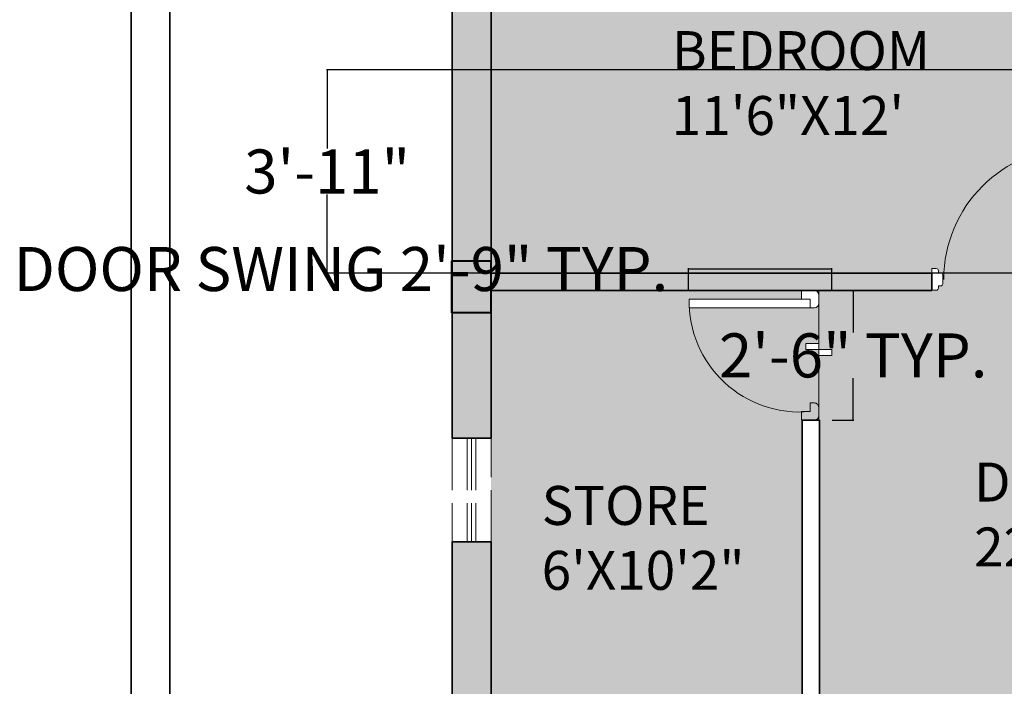
# Model space of a CAD drawing. Units: inches. Extents: x 1077 to 2505, y 1892 to 2728.
# Tile 11 of 26: x 1078 to 1306, y 2338 to 2492. Entities that reach past the tile are written whole.
import ezdxf

# ---------------------------------------------------------------- set-up
doc = ezdxf.new("R2010")
doc.units = ezdxf.units.IN
doc.linetypes.add('ACAD_ISO02W100', pattern=[15, 12, -3])
doc.layers.get('Defpoints').update_dxf_attribs({"color": 220, "linetype": 'ACAD_ISO02W100'})
for name, color, linetype, lineweight in [('00 FURNITURE', 15, 'Continuous', 15), ('A-ANNO-DIMS', 2, 'Continuous', 18), ('A-ANNO-TTLB', 7, 'Continuous', 35), ('A-AREA-IDEN', 7, 'Continuous', 18), ('A-COLS', 7, 'Continuous', 40), ('A-DOOR', 4, 'Continuous', 18), ('A-GLAZ-VENT', 6, 'ACAD_ISO02W100', 13), ('A-WALL-PATT', 7, 'Continuous', 9), ('A_FUR 1', 5, 'Continuous', 5), ('WALL', 7, 'Continuous', 35)]:
    doc.layers.add(name, color=color, linetype=linetype, lineweight=lineweight)
doc.layers.add('A-FLOR-PATT', color=254, linetype='Continuous', lineweight=9, true_color=0xd7ebd2)
doc.styles.get("Standard").update_dxf_attribs({"font": 'arial.ttf'})
doc.dimstyles.get("Standard").update_dxf_attribs({"dimtxt": 10.18, "dimasz": 0.18, "dimexe": 0.18, "dimexo": 0.0625, "dimgap": 0.09, "dimtad": 0, "dimtih": 1, "dimtoh": 1, "dimdec": 0, "dimzin": 0, "dimdsep": 46, "dimlunit": 3, "dimtxsty": 'Standard', "dimcen": 0.09, "dimadec": 0, "dimazin": 0, "dimtfac": 1, "dimtdec": 0, "dimtofl": 0, "dimtmove": 0, "dimatfit": 3, "dimfxl": 1, "dimtolj": 1, "dimtzin": 0, "dimarcsym": 0})

# ---------------------------------------------------------------- blocks, each defined once
blk = doc.blocks.new('DDD')
at = {"layer": '00 FURNITURE'}
for p, q in [((-12579.77, -15859.53), (-12579.77, -15829.05)), ((-12578.77, -15859.53), (-12578.77, -15829.03)), ((-12612.02, -15857.03), (-12612.02, -15862.03)), ((-12611.02, -15857.03), (-12612.02, -15857.03)), ((-12577.02, -15857.03), (-12576.02, -15857.03)), ((-12576.02, -15857.03), (-12576.02, -15862.03)), ((-12610.52, -15858.03), (-12610.52, -15857.53)), ((-12578.77, -15859.53), (-12579.77, -15859.53)), ((-12577.52, -15858.03), (-12577.52, -15857.53)), ((-12610.52, -15861.53), (-12610.52, -15861.03)), ((-12577.52, -15861.53), (-12577.52, -15861.03)), ((-12612.02, -15862.03), (-12611.02, -15862.03)), ((-12576.02, -15862.03), (-12577.02, -15862.03))]:
    blk.add_line(p, q, dxfattribs=at)
for points in [[(-12610.52, -15861.03), (-12610.02, -15861.03, 0.414214), (-12609.52, -15860.53), (-12609.52, -15858.53, 0.414214), (-12610.02, -15858.03), (-12610.52, -15858.03)], [(-12577.52, -15861.03), (-12578.02, -15861.03, -0.414214), (-12578.52, -15860.53), (-12578.52, -15858.53, -0.414214), (-12578.02, -15858.03), (-12577.52, -15858.03)]]:
    blk.add_lwpolyline(points, format="xyb", dxfattribs=at)
for centre, radius, start, end in [((-12578.77, -15859.53), 30.5, 90, 180), ((-12611.02, -15857.53), 0.5, 0, 90), ((-12577.02, -15857.53), 0.5, 90, 180), ((-12611.02, -15861.53), 0.5, 270, 0), ((-12577.02, -15861.53), 0.5, 180, 270)]:
    blk.add_arc(centre, radius, start, end, dxfattribs=at)
blk = doc.blocks.new('ESTSET')
at = {"layer": 'A_FUR 1'}
for p, q in [((-10.44, 4.1), (-10.44, 32.1)), ((-8.44, 4.1), (-8.44, 32.1)), ((-36.44, 6.1), (-36.44, 3.1)), ((-34.44, 6.1), (-36.44, 6.1)), ((-34.44, 4.1), (-34.44, 6.1)), ((-34.44, 4.1), (-34.44, 6.1)), ((-8.44, 4.1), (-8.44, 6.1)), ((-8.44, 6.1), (-6.44, 6.1)), ((-8.44, 4.1), (-8.44, 6.1)), ((-6.44, 6.1), (-6.44, 3.1)), ((-32.44, 4.1), (-34.44, 4.1)), ((-32.44, 4.1), (-34.44, 4.1)), ((-32.44, 3.1), (-32.44, 4.1)), ((-10.44, 3.1), (-10.44, 4.1)), ((-10.44, 4.1), (-8.44, 4.1)), ((-10.44, 4.1), (-8.44, 4.1)), ((-6.44, 2.1), (-36.44, 2.1)), ((-35.44, 2.1), (-33.44, 2.1)), ((-7.44, 2.1), (-9.44, 2.1))]:
    blk.add_line(p, q, dxfattribs=at)
for points in [[(-21.44, 2.1), (-18.67, 2.1), (-18.67, 5.1), (-20.06, 5.1)], [(-20.06, 5.1), (-20.06, -0.91)], [(-21.44, 2.1), (-21.44, -0.91), (-20.06, -0.91)]]:
    blk.add_lwpolyline(points, dxfattribs=at)
for centre, radius, start, end in [((-8.91, 6.46), 25.64, 88.9606, 185.2816), ((-35.44, 3.1), 1, 180, 270), ((-33.44, 3.1), 1, 270, 0), ((-9.44, 3.1), 1, 180, 270), ((-7.44, 3.1), 1, 270, 0)]:
    blk.add_arc(centre, radius, start, end, dxfattribs=at)
blk = doc.blocks.new('C1')
h = blk.add_hatch(color=256)
h.dxf.hatch_style = 1
h.paths.add_polyline_path([(1668.56, 2445.41), (1677.56, 2445.41), (1677.56, 2457.41), (1668.56, 2457.41)])
for p, q in [((1668.56, 2457.41), (1677.56, 2457.41)), ((1668.56, 2445.41), (1668.56, 2457.41)), ((1677.56, 2457.41), (1677.56, 2445.41)), ((1677.56, 2445.41), (1668.56, 2445.41))]:
    blk.add_line(p, q)
blk = doc.blocks.new('VENT-24')
for p, q in [((3.5, 24), (3.5, 0)), ((4.5, 24), (4.5, 0)), ((5.5, 24), (5.5, 0))]:
    blk.add_line(p, q)
blk.add_lwpolyline([(0, 0), (9, 0), (9, 24), (0, 24)], close=True)
blk = doc.blocks.new('SHEET-FRAME-RESIDENTIAL')
for points in [[(0, 830.04), (543.52, 830.04), (543.52, 0), (0, 0)], [(9, 821.04), (534.52, 821.04), (534.52, 9), (9, 9)]]:
    blk.add_lwpolyline(points, close=True)
blk = doc.blocks.new('*D34')
at = {"layer": 'A-ANNO-DIMS', "color": 0, "lineweight": -2, "transparency": 16777216}
for p, q in [((1233.24, 2434.11), (1233.06, 2434.11)), ((1233.24, 2429.21), (1233.24, 2434.29)), ((1266.19, 2434.11), (1233.42, 2434.11)), ((1266.37, 2429.21), (1266.37, 2434.29))]:
    blk.add_line(p, q, dxfattribs=at)
at = {"layer": 'A-ANNO-DIMS', "color": 0, "transparency": 16777216}
for points in [[(1233.42, 2434.14), (1233.42, 2434.08), (1233.24, 2434.11)], [(1266.19, 2434.14), (1266.19, 2434.08), (1266.37, 2434.11)]]:
    blk.add_solid(points, dxfattribs=at)
at = {"layer": 'Defpoints', "color": 0, "transparency": 16777216}
for p in [(1233.24, 2434.11), (1233.24, 2429.14), (1266.37, 2429.14)]:
    blk.add_point(p, dxfattribs=at)
at = {"layer": 'A-ANNO-DIMS', "color": 0, "transparency": 16777216, "insert": (1152.81, 2434.11), "char_height": 10.18, "attachment_point": 5}
blk.add_mtext('\\A1;DOOR SWING 2\'-9" TYP.', dxfattribs=at)
blk = doc.blocks.new('*D35')
at = {"layer": 'A-ANNO-DIMS', "color": 0, "lineweight": -2, "transparency": 16777216}
for p, q in [((1266.44, 2429.14), (1271.52, 2429.14)), ((1271.34, 2428.96), (1271.34, 2419.43)), ((1271.34, 2399.32), (1271.34, 2408.86)), ((1266.44, 2399.14), (1271.52, 2399.14))]:
    blk.add_line(p, q, dxfattribs=at)
at = {"layer": 'A-ANNO-DIMS', "color": 0, "transparency": 16777216}
for points in [[(1271.31, 2428.96), (1271.37, 2428.96), (1271.34, 2429.14)], [(1271.31, 2399.32), (1271.37, 2399.32), (1271.34, 2399.14)]]:
    blk.add_solid(points, dxfattribs=at)
at = {"layer": 'Defpoints', "color": 0, "transparency": 16777216}
for p in [(1266.37, 2429.14), (1271.34, 2429.14), (1266.37, 2399.14)]:
    blk.add_point(p, dxfattribs=at)
at = {"layer": 'A-ANNO-DIMS', "color": 0, "transparency": 16777216, "insert": (1271.34, 2414.14), "char_height": 10.18, "attachment_point": 5}
blk.add_mtext('\\A1;2\'-6" TYP.', dxfattribs=at)
blk = doc.blocks.new('*D64')
at = {"layer": 'A-ANNO-DIMS', "color": 0, "lineweight": -2, "transparency": 16777216}
for p, q in [((1395.47, 2480.16), (1149.43, 2480.16)), ((1149.61, 2479.98), (1149.61, 2461.95)), ((1149.61, 2433.34), (1149.61, 2451.37)), ((1395.47, 2433.16), (1149.43, 2433.16))]:
    blk.add_line(p, q, dxfattribs=at)
at = {"layer": 'A-ANNO-DIMS', "color": 0, "transparency": 16777216}
for points in [[(1149.58, 2479.98), (1149.64, 2479.98), (1149.61, 2480.16)], [(1149.58, 2433.34), (1149.64, 2433.34), (1149.61, 2433.16)]]:
    blk.add_solid(points, dxfattribs=at)
at = {"layer": 'Defpoints', "color": 0, "transparency": 16777216}
for p in [(1149.61, 2480.16), (1395.53, 2480.16), (1395.53, 2433.16)]:
    blk.add_point(p, dxfattribs=at)
at = {"layer": 'A-ANNO-DIMS', "color": 0, "transparency": 16777216, "insert": (1149.61, 2456.66), "char_height": 10.18, "attachment_point": 5}
blk.add_mtext('\\A1;3\'-11"', dxfattribs=at)

msp = doc.modelspace()

# ---------------------------------------------------------------- hatches: boundary and pattern name
at = {"layer": 'A-FLOR-PATT', "transparency": 33554559}
h = msp.add_hatch(color=256, dxfattribs=at)
h.dxf.hatch_style = 1
h.paths.add_polyline_path([(1395.53, 2577.16), (1374.83, 2577.16), (1350.83, 2577.19), (1350.83, 2577.16), (1329.53, 2577.16), (1329.53, 2480.16), (1329.53, 2469.16), (1325.53, 2469.16), (1325.53, 2515.13), (1307.53, 2515.13), (1307.53, 2577.16), (1269.31, 2577.16), (1221.31, 2577.15), (1221.31, 2577.16), (1187.53, 2577.16), (1187.53, 2433.16), (1289.53, 2433.16), (1289.53, 2429.16), (1263.53, 2429.16), (1187.53, 2429.16), (1187.53, 2395.02), (1187.53, 2395.02), (1187.53, 2371.02), (1187.53, 2371.02), (1187.53, 2307.16), (1259.53, 2307.16), (1259.53, 2399.16), (1263.53, 2399.16), (1263.53, 2307.16), (1289.53, 2307.16), (1289.53, 2306.23), (1325.53, 2306.23), (1325.53, 2307.16), (1329.53, 2307.16), (1329.53, 2306.23), (1365.53, 2306.23), (1365.53, 2307.16), (1432.53, 2307.16), (1432.53, 2088.16), (1547.53, 2088.16), (1547.53, 2140.08), (1511.53, 2140.08), (1511.53, 2267.16), (1475.53, 2267.16), (1475.53, 2303.16), (1468.53, 2303.16), (1468.53, 2307.16), (1547.53, 2307.16), (1547.53, 2348.22), (1547.53, 2396.22), (1547.53, 2429.16), (1435.53, 2429.16), (1435.53, 2433.16), (1476.35, 2433.16), (1476.35, 2451.18), (1547.53, 2451.18), (1547.53, 2577.16), (1499.53, 2577.16), (1499.53, 2586.16), (1547.53, 2586.16), (1547.53, 2642.16), (1518.18, 2642.16), (1518.18, 2642.05), (1494.15, 2642.05), (1494.15, 2642.16), (1469.53, 2642.16), (1469.53, 2577.16), (1399.53, 2577.16), (1399.53, 2429.16), (1325.53, 2429.16), (1325.53, 2433.16), (1329.53, 2433.16), (1395.53, 2433.16), (1395.53, 2480.16), (1359.53, 2480.16), (1359.53, 2484.16), (1395.53, 2484.16)])
h.paths.add_polyline_path([(1357.65, 2482.07), (1355.65, 2482.07), (1355.65, 2481.07, 0.414214), (1356.65, 2480.07), (1344.65, 2480.07), (1344.65, 2477.06), (1343.27, 2477.06), (1343.27, 2480.07), (1330.65, 2480.07, -0.414214), (1329.65, 2481.07), (1329.65, 2484.07), (1331.65, 2484.07), (1331.65, 2510.07, -0.446908)], flags=16)
h.paths.add_polyline_path([(1305.09, 2559.18), (1288.89, 2559.18), (1288.89, 2575.38), (1305.09, 2575.38)], flags=16)
h.paths.add_polyline_path([(1304.19, 2560.08), (1289.79, 2560.08), (1289.79, 2574.48), (1304.19, 2574.48)], flags=0)
h.paths.add_polyline_path([(1287.99, 2500.68, -0.414214), (1287.09, 2499.78), (1265.14, 2499.78), (1224.09, 2499.78, -0.414214), (1223.19, 2500.68), (1223.19, 2557.16), (1223.19, 2571.74), (1223.19, 2575.38), (1287.99, 2575.38), (1287.99, 2571.74), (1287.09, 2571.74, -0.414214), (1287.99, 2570.84)], flags=16)
h.paths.add_polyline_path([(1292.98, 2569.05, -1), (1300.92, 2569.05, -1)], flags=0)
h.paths.add_polyline_path([(1293.32, 2569.05, -1), (1300.58, 2569.05, -1)], flags=0)
h.paths.add_polyline_path([(1322.8, 2462.21), (1322.8, 2431.71), (1323.05, 2430.71), (1323.05, 2431.71), (1321.8, 2431.71), (1321.8, 2462.19, 0.404641), (1292.3, 2431.71), (1292.05, 2430.71, -0.414214), (1291.55, 2430.21), (1291.05, 2430.21), (1291.05, 2429.71, -0.414214), (1290.55, 2429.21), (1289.55, 2429.21), (1289.55, 2434.21), (1290.55, 2434.21, -0.414214), (1291.05, 2433.71), (1291.05, 2433.21), (1291.55, 2433.21, -0.414214), (1292.05, 2432.71), (1292.3, 2431.71, -0.414214)], flags=16)
h.paths.add_polyline_path([(1287.82, 2548.28, 0.292232), (1279.17, 2536.8, 0.052719), (1223.93, 2548.28), (1223.28, 2548.28), (1223.28, 2557.16), (1223.93, 2557.16), (1245.42, 2557.16, -0.117785), (1245.77, 2557.93, -0.059418), (1254.87, 2567.02, -0.379859), (1257.28, 2566.88, -0.02509), (1261.41, 2563.32, -0.025935), (1265.65, 2567.02, -0.379859), (1268.06, 2566.88, -0.061767), (1277.52, 2557.43, -0.069393), (1277.82, 2557.16), (1287.82, 2557.16)], flags=0)
h.paths.add_polyline_path([(1263.47, 2548.28), (1260.56, 2548.28, -0.015371), (1258.01, 2546.13, -0.429576), (1255.37, 2546.06, -0.016036), (1252.69, 2548.28), (1223.28, 2548.28), (1223.28, 2554.42), (1246.78, 2554.42, 0.055344), (1255.37, 2546.06, 0.331768), (1257.52, 2545.74, 0.027343), (1262, 2549.64, 0.00919)], flags=0)
h.paths.add_polyline_path([(1295.56, 2568.34), (1296.87, 2569.09), (1296.87, 2570.6, 0.399698), (1295.39, 2569.05, 0.119004)], flags=0)
h.paths.add_polyline_path([(1295.21, 2569.05, -1), (1298.68, 2569.05, -1)], flags=0)
h.paths.add_polyline_path([(1296.95, 2568.96), (1297.03, 2569), (1297.03, 2569.09), (1296.99, 2569.11), (1296.91, 2568.98)], flags=0)
h.paths.add_polyline_path([(1402.28, 2462.19, -0.414214), (1432.78, 2431.69), (1433.03, 2432.69), (1432.78, 2431.69, 0.404641), (1403.28, 2462.17), (1403.28, 2431.69), (1402.03, 2431.69), (1402.03, 2430.69, -0.414214), (1401.53, 2430.19), (1401.03, 2430.19), (1401.03, 2429.69, -0.414214), (1400.53, 2429.19), (1399.53, 2429.19), (1399.53, 2434.19), (1400.53, 2434.19, -0.414214), (1401.03, 2433.69), (1401.03, 2433.19), (1401.53, 2433.19, -0.414214), (1402.03, 2432.69)], flags=16)
h.paths.add_polyline_path([(1470.16, 2535.21, -0.414214), (1471.06, 2536.11), (1527.54, 2536.11), (1542.12, 2536.11), (1545.76, 2536.11), (1545.76, 2471.31), (1542.12, 2471.31), (1542.12, 2472.21, -0.414214), (1541.22, 2471.31), (1471.06, 2471.31, -0.414214), (1470.16, 2472.21), (1470.16, 2494.16)], flags=16)
h.paths.add_polyline_path([(1483.07, 2536.11, 0.253465), (1480.11, 2526.15, 0.2538), (1470.15, 2523.19)], flags=16)
h.paths.add_polyline_path([(1223.19, 2512.69, 0.253465), (1233.14, 2509.74, 0.2538), (1236.1, 2499.77)], flags=16)
h.paths.add_polyline_path([(1469.77, 2578.72), (1469.77, 2581.72), (1471.77, 2581.72), (1471.77, 2607.72, -0.01951), (1473.77, 2607.68), (1473.77, 2579.72), (1473.77, 2578.72, -0.414214), (1472.77, 2577.72), (1470.77, 2577.72, -0.414214)], flags=16)
h.paths.add_polyline_path([(1382.46, 2398.13), (1395.04, 2398.13), (1395.04, 2399.74), (1382.46, 2399.74)], flags=16)
h.paths.add_polyline_path([(1379.94, 2397.18), (1379.94, 2389.82), (1380.5, 2389.82), (1380.5, 2396.05, -0.41429), (1381.06, 2396.61), (1396.47, 2396.61, -0.414213), (1397.03, 2396.05), (1397.03, 2389.82), (1397.59, 2389.82), (1397.59, 2397.18)], flags=16)
h.paths.add_polyline_path([(1263.37, 2428.14), (1263.37, 2426.14, -0.414214), (1262.37, 2425.14), (1261.37, 2425.14), (1233.41, 2425.14, 0.400854), (1259.37, 2401.04), (1259.37, 2401.14), (1261.37, 2401.14, -0.446908), (1233.37, 2427.14), (1259.37, 2427.14), (1259.37, 2429.14), (1262.37, 2429.14, -0.414214)], flags=16)
h.paths.add_polyline_path([(1404.79, 2398.13), (1417.37, 2398.13), (1417.37, 2399.74), (1404.79, 2399.74)], flags=16)
h.paths.add_polyline_path([(1402.27, 2397.18), (1404.79, 2398.13), (1417.37, 2398.13), (1419.92, 2397.18)], flags=16)
h.paths.add_polyline_path([(1432.26, 2383.16), (1432.26, 2370.59), (1433.87, 2370.59), (1433.87, 2383.16)], flags=16)
h.paths.add_polyline_path([(1431.3, 2385.69), (1423.84, 2385.69), (1423.84, 2385.13), (1430.18, 2385.13, -0.41429), (1430.74, 2384.57), (1430.74, 2369.16, -0.414237), (1430.18, 2368.6), (1423.84, 2368.6), (1423.84, 2368.03), (1431.3, 2368.03)], flags=16)
h.paths.add_polyline_path([(1417.37, 2351.16), (1417.37, 2349.54), (1418.9, 2349.54, 0.414236), (1419.92, 2350.56), (1419.92, 2352.11)], flags=16)
h.paths.add_polyline_path([(1395.04, 2351.16), (1395.04, 2349.54), (1396.58, 2349.54, 0.414235), (1397.59, 2350.56), (1397.59, 2352.11)], flags=16)
h.paths.add_polyline_path([(1366.7, 2370.05), (1365.09, 2370.05), (1365.09, 2368.52, 0.414235), (1366.11, 2367.5), (1367.66, 2367.5)], flags=16)
h.paths.add_polyline_path([(1419.36, 2359.47), (1419.36, 2353.24, -0.41419), (1418.8, 2352.68), (1403.39, 2352.68, -0.414137), (1402.83, 2353.24), (1402.83, 2359.47), (1397.03, 2359.47), (1397.03, 2353.24, -0.414189), (1396.47, 2352.68), (1381.06, 2352.68, -0.414137), (1380.5, 2353.24), (1380.5, 2359.47)], flags=16)
h.paths.add_polyline_path([(1222.29, 2559.18), (1206.09, 2559.18), (1206.09, 2575.38), (1222.29, 2575.38)], flags=16)
h.paths.add_polyline_path([(1221.39, 2560.08), (1206.99, 2560.08), (1206.99, 2574.48), (1221.39, 2574.48)], flags=0)
h.paths.add_polyline_path([(1482, 2577.72), (1482, 2580.73), (1483.38, 2580.73), (1483.38, 2577.72), (1484.77, 2577.72), (1484.77, 2574.72), (1483.38, 2574.72), (1483.38, 2577.72)], flags=16)
h.paths.add_polyline_path([(1266.37, 2415.53), (1266.37, 2414.14), (1263.37, 2414.14), (1263.37, 2415.53), (1260.36, 2415.53), (1260.36, 2416.91), (1263.37, 2416.91), (1263.37, 2415.53)], flags=16)
h.paths.add_polyline_path([(1210.26, 2569.05, -1), (1218.19, 2569.05, -1)], flags=0)
h.paths.add_polyline_path([(1210.6, 2569.05, -1), (1217.85, 2569.05, -1)], flags=0)
h.paths.add_polyline_path([(1212.84, 2568.34), (1214.15, 2569.09), (1214.15, 2570.6, 0.399698), (1212.67, 2569.05, 0.119004)], flags=0)
h.paths.add_polyline_path([(1212.49, 2569.05, -1), (1215.96, 2569.05, -1)], flags=0)
h.paths.add_polyline_path([(1214.23, 2568.96), (1214.3, 2568.91), (1214.3, 2569)], flags=0)
h.paths.add_polyline_path([(1507.18, 2480.12, 0.052719), (1518.66, 2535.36), (1518.66, 2536.01), (1527.54, 2536.01), (1527.54, 2535.36), (1527.54, 2513.88, -0.117785), (1528.31, 2513.53, -0.059418), (1537.4, 2504.43, -0.379859), (1537.26, 2502.01, -0.02509), (1533.7, 2497.89, -0.025935), (1537.4, 2493.64, -0.379859), (1537.26, 2491.23, -0.061767), (1527.8, 2481.77, -0.069393), (1527.54, 2481.47), (1527.54, 2471.47), (1518.66, 2471.47, 0.292232)], flags=0)
h.paths.add_polyline_path([(1516.43, 2503.92, -0.016036), (1518.66, 2506.6), (1518.66, 2536.01), (1524.8, 2536.01), (1524.8, 2512.51, 0.055344), (1516.43, 2503.92, 0.331768), (1516.12, 2501.77, 0.027343), (1520.01, 2497.29, 0.00919), (1518.66, 2495.82), (1518.66, 2498.73, -0.015371), (1516.5, 2501.28, -0.429576)], flags=0)
h.paths.add_polyline_path([(1499.63, 2625.5, -0.171636), (1502.82, 2631.01), (1502.82, 2633.37), (1498.68, 2633.37, -0.414214), (1497.7, 2634.36), (1497.7, 2640.66, -0.414214), (1498.68, 2641.64), (1514.82, 2641.64, -0.414214), (1515.81, 2640.66), (1515.81, 2634.36, -0.414214), (1514.82, 2633.37), (1510.69, 2633.37), (1510.69, 2631.01, -0.171636), (1513.88, 2625.5, -0.258205), (1509.31, 2614.47), (1504.19, 2614.47, -0.258205)], flags=16)
h.paths.add_polyline_path([(1501.2, 2625.5, -0.171636), (1504.39, 2631.01), (1509.12, 2631.01, -0.171636), (1512.3, 2625.5, -0.210384), (1509.35, 2616.02), (1504.16, 2616.02, -0.210384)], flags=0)
h.paths.add_polyline_path([(1529.56, 2537.01), (1529.56, 2553.21), (1545.76, 2553.21), (1545.76, 2537.01)], flags=16)
h.paths.add_polyline_path([(1530.46, 2537.91), (1530.46, 2552.31), (1544.86, 2552.31), (1544.86, 2537.91)], flags=0)
h.paths.add_polyline_path([(1535.45, 2545.07, -1), (1543.39, 2545.07, -1)], flags=0)
h.paths.add_polyline_path([(1535.8, 2545.07, -1), (1543.05, 2545.07, -1)], flags=0)
h.paths.add_polyline_path([(1529.56, 2470.41), (1545.76, 2470.41), (1545.76, 2454.21), (1529.56, 2454.21)], flags=16)
h.paths.add_polyline_path([(1541.16, 2544.99), (1540.98, 2544.99, -0.544606), (1538.71, 2543.68), (1538.62, 2543.53, 0.547962)], flags=0)
h.paths.add_polyline_path([(1530.46, 2469.51), (1544.86, 2469.51), (1544.86, 2455.11), (1530.46, 2455.11)], flags=0)
h.paths.add_polyline_path([(1539.47, 2545.14), (1539.42, 2545.22), (1539.38, 2545.14)], flags=0)
h.paths.add_polyline_path([(1543.39, 2462.34, -1), (1535.45, 2462.34, -1)], flags=0)
h.paths.add_polyline_path([(1543.05, 2462.34, -1), (1535.8, 2462.34, -1)], flags=0)
h.paths.add_polyline_path([(1541.16, 2462.27), (1540.98, 2462.27, -0.544606), (1538.71, 2460.96), (1538.62, 2460.8, 0.547962)], flags=0)
h.paths.add_polyline_path([(1539.47, 2462.42), (1539.42, 2462.5), (1539.38, 2462.42)], flags=0)
h.paths.add_polyline_path([(1435.32, 2335.25, -0.414214), (1465.82, 2304.75), (1466.07, 2305.75), (1465.82, 2304.75, 0.404641), (1436.32, 2335.23), (1436.32, 2304.75), (1435.07, 2304.75), (1435.07, 2303.75, -0.414214), (1434.57, 2303.25), (1434.07, 2303.25), (1434.07, 2302.75, -0.414214), (1433.57, 2302.25), (1432.57, 2302.25), (1432.57, 2307.25), (1433.57, 2307.25, -0.414214), (1434.07, 2306.75), (1434.07, 2306.25), (1434.57, 2306.25, -0.414214), (1435.07, 2305.75)], flags=16)
h.paths.add_polyline_path([(1532.13, 2635.71), (1535.43, 2635.71), (1535.43, 2635.89), (1532.13, 2635.89)], flags=16)
edge = h.paths.add_edge_path(flags=16)
edge.add_arc((1535.98, 2632.67), 0.183, 270, 360)
edge.add_line((1536.17, 2632.67), (1536.17, 2639.82))
edge.add_line((1536.17, 2639.82), (1538.29, 2639.82))
edge.add_line((1538.29, 2639.82), (1538.29, 2641.82))
edge.add_line((1538.29, 2641.82), (1533.25, 2641.82))
edge.add_line((1533.25, 2641.82), (1533.25, 2639.82))
edge.add_line((1533.25, 2639.82), (1534.87, 2639.82))
edge.add_line((1534.87, 2639.82), (1534.87, 2639))
edge.add_line((1534.87, 2639), (1533.7, 2639))
edge.add_line((1533.7, 2639), (1533.7, 2639.82))
edge.add_line((1533.7, 2639.82), (1533.25, 2639.82))
edge.add_line((1533.25, 2639.82), (1533.25, 2641.82))
edge.add_line((1533.25, 2641.82), (1538.29, 2641.82))
edge.add_line((1538.29, 2641.82), (1538.29, 2641.34))
edge.add_line((1538.29, 2641.34), (1540.64, 2641.58))
edge.add_line((1540.64, 2641.58), (1540.64, 2641.82))
edge.add_line((1540.64, 2641.82), (1541.5, 2641.82))
edge.add_line((1541.5, 2641.82), (1541.5, 2641.25))
edge.add_line((1541.5, 2641.25), (1541.31, 2639.79))
edge.add_ellipse((1541.09, 2638.95), major_axis=(-1.08, 0), ratio=0.790849, start_angle=180, end_angle=255.2976, ccw=False)
edge.add_line((1542.17, 2638.95), (1542.17, 2638.38))
edge.add_ellipse((1541.09, 2638.38), major_axis=(-1.08, 0), ratio=0.790849, start_angle=0, end_angle=180, ccw=False)
edge.add_line((1540, 2638.38), (1540.01, 2638.87))
edge.add_ellipse((1541.09, 2638.95), major_axis=(-1.08, 0), ratio=0.790849, start_angle=284.7024, end_angle=364.0401, ccw=False)
edge.add_line((1540.78, 2639.75), (1540.78, 2641.25))
edge.add_line((1540.78, 2641.25), (1540.64, 2641.25))
edge.add_line((1540.64, 2641.25), (1538.29, 2641.01))
edge.add_line((1538.29, 2641.01), (1538.29, 2639.82))
edge.add_line((1538.29, 2639.82), (1536.17, 2639.82))
edge.add_line((1536.17, 2639.82), (1536.17, 2632.48))
edge.add_line((1536.17, 2632.48), (1535.98, 2632.48))
h.paths.add_polyline_path([(1496.32, 2250.34, -0.292371), (1498.9, 2247.83, -0.085148), (1501.21, 2208.85, -0.01331), (1500.27, 2098.5, -0.379287), (1497.22, 2095.28, -0.0502), (1441.54, 2095.28, -0.379287), (1438.5, 2098.5, -0.01331), (1437.56, 2208.85, -0.086132), (1439.96, 2248.26, -0.295116), (1442.59, 2250.78, -0.114238)], flags=16)
h.paths.add_polyline_path([(1495.16, 2205.84, -0.355389), (1496.7, 2202.1), (1492.94, 2189.65, -0.398275), (1489.12, 2187.47, 0.113332), (1449.64, 2187.47, -0.398275), (1445.82, 2189.65), (1442.06, 2202.1, -0.355394), (1443.6, 2205.84, -0.265725)], flags=0)
h.paths.add_polyline_path([(1440.37, 2195.72), (1445.94, 2181.67), (1445.94, 2160.63), (1440.84, 2157.26)], flags=0)
h.paths.add_polyline_path([(1498.46, 2195.72), (1497.99, 2157.26), (1492.88, 2160.63), (1492.88, 2181.67)], flags=0)
h.paths.add_polyline_path([(1445.94, 2158.37), (1445.94, 2137.12), (1441.12, 2122.56), (1440.87, 2155.03)], flags=0)
h.paths.add_polyline_path([(1492.88, 2158.37), (1497.96, 2155.03), (1497.71, 2122.56), (1492.88, 2137.12)], flags=0)
h.paths.add_polyline_path([(1489.88, 2130.4), (1494.39, 2107.67, -0.090102), (1444.44, 2107.65), (1448.95, 2130.39, 0.036636)], flags=0)
h.paths.add_polyline_path([(1447.54, 2159.34), (1497.44, 2159.34), (1497.44, 2177.89), (1447.54, 2177.89)], flags=8)
h.paths.add_polyline_path([(1196.44, 2354.84), (1246.65, 2354.84), (1246.65, 2388.43), (1196.44, 2388.43)], flags=24)
h.paths.add_polyline_path([(1296.09, 2360.25), (1353.81, 2360.25), (1353.81, 2393.84), (1296.09, 2393.84)], flags=24)
h.paths.add_polyline_path([(1400.72, 2471.85), (1470.63, 2471.85), (1470.63, 2505.44), (1400.72, 2505.44)], flags=24)
h.paths.add_polyline_path([(1324.78, 2448.48), (1394.95, 2448.48), (1394.95, 2467.02), (1324.78, 2467.02)], flags=24)
h.paths.add_polyline_path([(1335.08, 2531.43), (1389.67, 2531.43), (1389.67, 2565.02), (1335.08, 2565.02)], flags=24)
h.paths.add_polyline_path([(1225.76, 2460), (1295.67, 2460), (1295.67, 2493.58), (1225.76, 2493.58)], flags=24)
h = msp.add_hatch(color=256, dxfattribs=at)
h.dxf.hatch_style = 1
h.paths.add_polyline_path([(1547.53, 2348.22), (1547.53, 2396.22), (1547.53, 2425.11), (1547.53, 2425.11), (1547.53, 2429.16), (1435.53, 2429.16), (1434.03, 2429.21), (1434.03, 2430.19), (1433.03, 2430.19), (1432.78, 2431.69, 0.404641), (1403.28, 2462.17), (1403.28, 2431.69), (1402.03, 2431.69), (1402.03, 2430.19), (1401.03, 2430.19), (1401.03, 2429.19), (1399.53, 2429.19), (1399.53, 2429.19), (1399.53, 2429.16), (1334.67, 2429.16), (1334.67, 2423.95), (1325.67, 2423.95), (1325.67, 2429.16), (1325.53, 2429.16), (1324.05, 2429.24), (1324.05, 2430.21), (1323.05, 2430.21), (1323.05, 2431.71), (1321.8, 2431.71), (1321.8, 2462.19, 0.416544), (1292.05, 2430.73, -0.423614), (1291.55, 2430.21), (1291.05, 2430.21), (1291.05, 2429.21), (1289.55, 2429.21), (1289.53, 2429.21), (1289.53, 2429.16), (1263.37, 2429.16), (1263.37, 2415.53), (1266.37, 2415.53), (1266.37, 2414.14), (1263.37, 2414.14), (1263.37, 2399.16), (1263.53, 2399.16), (1263.53, 2307.16), (1289.53, 2307.16), (1289.53, 2306.23), (1323.26, 2306.23), (1323.26, 2307.21), (1332.26, 2307.21), (1365.53, 2306.23), (1365.53, 2307.16), (1432.53, 2307.16), (1432.57, 2307.16), (1432.57, 2307.25), (1434.07, 2307.25), (1434.07, 2306.25), (1435.32, 2306.25), (1435.32, 2335.25, -0.407346), (1466.07, 2305.73, -0.423614), (1466.57, 2306.25), (1467.07, 2306.25), (1467.07, 2307.25), (1468.57, 2307.25), (1547.53, 2307.16), (1547.53, 2307.2)])
h.paths.add_polyline_path([(1430.74, 2369.16), (1430.74, 2384.57, 0.41429), (1430.18, 2385.13), (1423.84, 2385.13), (1423.84, 2368.6), (1430.18, 2368.6, 0.414237)], flags=16)
h.paths.add_polyline_path([(1432.26, 2383.16), (1432.26, 2370.59), (1433.87, 2370.59), (1433.87, 2383.16)], flags=16)
h.paths.add_polyline_path([(1431.3, 2368.03), (1431.3, 2385.69), (1432.26, 2383.16), (1432.26, 2370.59)], flags=16)
h.paths.add_polyline_path([(1417.37, 2351.16), (1417.37, 2349.54), (1418.9, 2349.54, 0.414236), (1419.92, 2350.56), (1419.92, 2352.11)], flags=16)
h.paths.add_polyline_path([(1403.39, 2352.68), (1418.78, 2352.68, 0.42427), (1419.36, 2353.24), (1419.36, 2359.47), (1402.83, 2359.47), (1402.83, 2353.24, 0.414137)], flags=16)
h.paths.add_polyline_path([(1366.7, 2370.05), (1365.09, 2370.05), (1365.09, 2368.52, 0.414235), (1366.11, 2367.5), (1367.66, 2367.5)], flags=16)
h.paths.add_polyline_path([(1382.46, 2398.13), (1395.04, 2398.13), (1395.04, 2399.74), (1382.46, 2399.74)], flags=16)
h.paths.add_polyline_path([(1396.47, 2396.61), (1381.06, 2396.61, 0.41429), (1380.5, 2396.05), (1380.5, 2389.82), (1397.03, 2389.82), (1397.03, 2396.05, 0.414213)], flags=16)
h.paths.add_polyline_path([(1402.27, 2397.18), (1402.83, 2396.05, -0.414213), (1403.39, 2396.61)], flags=16)
h.paths.add_polyline_path([(1418.8, 2396.61), (1419.36, 2396.61), (1419.36, 2396.05, 0.414237)], flags=16)
h.paths.add_polyline_path([(1404.79, 2398.13), (1417.37, 2398.13), (1417.37, 2399.74), (1404.79, 2399.74)], flags=16)
h.paths.add_polyline_path([(1381.06, 2352.68, -0.414213), (1380.5, 2353.24), (1380.27, 2352.11)], flags=16)
h.paths.add_polyline_path([(1396.58, 2349.54), (1396.58, 2349.54), (1395.04, 2349.54), (1395.04, 2349.54), (1382.46, 2349.54), (1382.46, 2351.16), (1395.04, 2351.16), (1397.59, 2352.11), (1397.59, 2350.56, -0.414235)], flags=16)
h.paths.add_polyline_path([(1379.94, 2397.18), (1382.46, 2398.13), (1395.04, 2398.13), (1397.59, 2397.18)], flags=16)
h.paths.add_polyline_path([(1368.78, 2384.59, 0.414213), (1368.22, 2384.03), (1367.66, 2367.5), (1367.66, 2385.15)], flags=16)
h.paths.add_polyline_path([(1547.53, 2574.38), (1547.51, 2574.38), (1547.51, 2577.16), (1499.53, 2577.16), (1484.77, 2577.44), (1484.77, 2574.72), (1483.38, 2574.72), (1483.38, 2577.72), (1482, 2577.72), (1469.53, 2577.72), (1469.53, 2577.16), (1401.95, 2577.16), (1401.95, 2574.12), (1399.53, 2574.12), (1399.53, 2434.19), (1401.03, 2434.19), (1401.03, 2433.19), (1402.28, 2433.19), (1402.28, 2462.19, -0.407346), (1433.03, 2432.67, -0.423614), (1433.53, 2433.19), (1434.03, 2433.19), (1434.03, 2434.19), (1435.53, 2434.19), (1476.35, 2433.81), (1476.35, 2451.18), (1547.53, 2451.18)])
h.paths.add_polyline_path([(1470.16, 2535.21, -0.414214), (1471.06, 2536.11), (1527.54, 2536.11), (1542.12, 2536.11), (1545.76, 2536.11), (1545.76, 2471.31), (1542.12, 2471.31), (1542.12, 2472.21, -0.414214), (1541.22, 2471.31), (1471.06, 2471.31, -0.414214), (1470.16, 2472.21), (1470.16, 2494.16)], flags=16)
h.paths.add_polyline_path([(1483.07, 2536.11, 0.253465), (1480.11, 2526.15, 0.2538), (1470.15, 2523.19)], flags=16)
h.paths.add_polyline_path([(1525.55, 2481.52, -0.000893), (1524.8, 2482.24), (1524.8, 2471.47), (1527.54, 2471.47), (1527.54, 2472.12), (1527.54, 2481.47, -0.388819)], flags=0)
h.paths.add_polyline_path([(1518.66, 2536.01), (1527.54, 2536.01), (1527.54, 2535.36), (1527.54, 2513.88, -0.117785), (1528.31, 2513.53, -0.059418), (1537.4, 2504.43, -0.379859), (1537.26, 2502.01, -0.02509), (1533.7, 2497.89, 0.033431), (1528.3, 2502.74, 0.308459), (1526.25, 2502.88, 0.047827), (1518.66, 2495.82), (1518.66, 2498.73, -0.015371), (1516.5, 2501.28, -0.429576), (1516.43, 2503.92, -0.016036), (1518.66, 2506.6)], flags=0)
h.paths.add_polyline_path([(1529.56, 2537.01), (1529.56, 2553.21), (1545.76, 2553.21), (1545.76, 2537.01)], flags=16)
h.paths.add_polyline_path([(1530.46, 2537.91), (1530.46, 2552.31), (1544.86, 2552.31), (1544.86, 2537.91)], flags=0)
h.paths.add_polyline_path([(1535.8, 2545.07, -1), (1543.05, 2545.07, -1)], flags=0)
h.paths.add_polyline_path([(1541.16, 2544.99), (1540.98, 2544.99, -0.544606), (1538.71, 2543.68), (1538.62, 2543.53, 0.547962)], flags=0)
h.paths.add_polyline_path([(1539.47, 2545.14), (1539.42, 2545.22), (1539.38, 2545.14)], flags=0)
h.paths.add_polyline_path([(1529.56, 2470.41), (1545.76, 2470.41), (1545.76, 2454.21), (1529.56, 2454.21)], flags=16)
h.paths.add_polyline_path([(1530.46, 2469.51), (1544.86, 2469.51), (1544.86, 2455.11), (1530.46, 2455.11)], flags=0)
h.paths.add_polyline_path([(1535.8, 2462.34, -1), (1543.05, 2462.34, -1)], flags=0)
h.paths.add_polyline_path([(1541.16, 2462.27), (1540.98, 2462.27, -0.544606), (1538.71, 2460.96), (1538.62, 2460.8, 0.547962)], flags=0)
h.paths.add_polyline_path([(1539.47, 2462.42), (1539.42, 2462.5), (1539.38, 2462.42)], flags=0)
h.paths.add_polyline_path([(1395.53, 2574.12), (1392.95, 2574.12), (1392.95, 2577.16), (1374.83, 2577.16), (1350.83, 2577.19), (1350.83, 2577.16), (1332.07, 2577.16), (1332.07, 2574), (1329.53, 2574), (1329.53, 2484.07), (1331.65, 2484.07), (1331.65, 2510.07, -0.423677), (1357.76, 2484.07), (1359.53, 2484.07), (1359.53, 2484.16), (1395.53, 2484.16)], flags=17)
h.paths.add_polyline_path([(1395.53, 2480.16), (1359.06, 2480.16, 0.437533), (1359.53, 2481.55), (1359.53, 2484.16), (1395.53, 2484.16), (1395.53, 2574.12), (1392.95, 2574.12), (1392.95, 2577.16), (1374.83, 2577.16), (1350.83, 2577.19), (1350.83, 2577.16), (1332.07, 2577.16), (1332.07, 2574), (1329.53, 2574), (1329.53, 2484.07), (1329.65, 2484.07), (1329.65, 2481.07), (1329.53, 2480.16), (1329.53, 2469.16), (1325.53, 2469.16), (1325.53, 2515.13), (1307.53, 2515.13), (1307.53, 2577.16), (1269.31, 2577.16), (1221.31, 2577.15), (1221.31, 2577.16), (1187.61, 2577.16), (1187.61, 2574.03), (1187.53, 2433.16), (1289.55, 2433.16), (1289.55, 2434.21), (1291.05, 2434.21), (1291.05, 2433.21), (1292.05, 2433.21), (1292.3, 2431.71, -0.414214), (1322.8, 2462.21), (1323.05, 2432.71, -0.414214), (1323.55, 2433.21), (1324.05, 2433.21), (1324.05, 2434.21), (1325.67, 2434.21), (1325.67, 2435.95), (1334.67, 2435.95), (1334.67, 2433.16), (1395.53, 2433.16)])
h.paths.add_polyline_path([(1344.65, 2480.07), (1344.65, 2477.06), (1343.27, 2477.06), (1343.27, 2480.07), (1332.65, 2480.07, 0.414214), (1333.65, 2481.07), (1333.65, 2482.07), (1331.65, 2482.07), (1331.65, 2484.07), (1331.65, 2510.07, -0.446908), (1357.65, 2482.07), (1355.65, 2482.07), (1355.65, 2481.07, 0.414214), (1356.65, 2480.07)], flags=16)
h.paths.add_polyline_path([(1287.99, 2500.68, -0.414214), (1287.09, 2499.78), (1265.14, 2499.78), (1224.09, 2499.78, -0.414214), (1223.19, 2500.68), (1223.19, 2557.16), (1223.19, 2571.74), (1223.19, 2575.38), (1287.99, 2575.38), (1287.99, 2571.74), (1287.09, 2571.74, -0.414214), (1287.99, 2570.84)], flags=16)
h.paths.add_polyline_path([(1277.77, 2555.17, -0.000893), (1277.05, 2554.42), (1287.82, 2554.42), (1287.82, 2557.16), (1287.17, 2557.16), (1277.82, 2557.16, -0.388819)], flags=0)
h.paths.add_polyline_path([(1223.28, 2548.28), (1223.28, 2557.16), (1223.93, 2557.16), (1245.42, 2557.16, -0.117785), (1245.77, 2557.93, -0.059418), (1254.87, 2567.02, -0.379859), (1257.28, 2566.88, -0.02509), (1261.41, 2563.32, 0.033431), (1256.55, 2557.93, 0.308459), (1256.41, 2555.88, 0.047827), (1263.47, 2548.28), (1260.56, 2548.28, -0.015371), (1258.01, 2546.13, -0.429576), (1255.37, 2546.06, -0.016036), (1252.69, 2548.28)], flags=0)
h.paths.add_polyline_path([(1305.09, 2559.18), (1288.89, 2559.18), (1288.89, 2575.38), (1305.09, 2575.38)], flags=16)
h.paths.add_polyline_path([(1304.19, 2560.08), (1289.79, 2560.08), (1289.79, 2574.48), (1304.19, 2574.48)], flags=0)
h.paths.add_polyline_path([(1300.58, 2569.05, -1), (1293.32, 2569.05, -1)], flags=0)
h.paths.add_polyline_path([(1223.19, 2512.69, 0.253465), (1233.14, 2509.74, 0.2538), (1236.1, 2499.77)], flags=16)
h.paths.add_polyline_path([(1295.56, 2568.34), (1296.87, 2569.09), (1296.87, 2570.6, 0.399698), (1295.39, 2569.05, 0.119004)], flags=0)
h.paths.add_polyline_path([(1295.21, 2569.05, -1), (1298.68, 2569.05, -1)], flags=0)
h.paths.add_polyline_path([(1296.95, 2568.96), (1297.03, 2569), (1297.03, 2569.09), (1296.99, 2569.11), (1296.91, 2568.98)], flags=0)
h.paths.add_polyline_path([(1222.29, 2559.18), (1206.09, 2559.18), (1206.09, 2575.38), (1222.29, 2575.38)], flags=16)
h.paths.add_polyline_path([(1221.39, 2560.08), (1206.99, 2560.08), (1206.99, 2574.48), (1221.39, 2574.48)], flags=0)
h.paths.add_polyline_path([(1217.85, 2569.05, -1), (1210.6, 2569.05, -1)], flags=0)
h.paths.add_polyline_path([(1212.84, 2568.34), (1214.15, 2569.09), (1214.15, 2570.6, 0.399698), (1212.67, 2569.05, 0.119004)], flags=0)
h.paths.add_polyline_path([(1212.49, 2569.05, -1), (1215.96, 2569.05, -1)], flags=0)
h.paths.add_polyline_path([(1214.23, 2568.96), (1214.3, 2569), (1214.3, 2569.09), (1214.26, 2569.11), (1214.19, 2568.98)], flags=0)
h.paths.add_polyline_path([(1259.53, 2399.14), (1259.37, 2399.14), (1259.37, 2401.04, -0.423677), (1233.37, 2427.14), (1259.37, 2427.14), (1259.37, 2429.16), (1187.53, 2429.16), (1187.53, 2395.02), (1187.53, 2395.02), (1187.53, 2371.02), (1187.53, 2371.02), (1187.53, 2311.49), (1187.55, 2311.49), (1187.55, 2307.16), (1259.53, 2307.16)])
h.paths.add_polyline_path([(1323.26, 2295.21), (1323.26, 2304.23), (1289.53, 2304.23), (1289.53, 2303.16), (1187.55, 2303.16), (1187.55, 2299.49), (1178.53, 2299.49), (1178.53, 2267.66), (1178.53, 2219.66), (1182.03, 2219.66), (1182.03, 2267.67), (1184.03, 2267.67), (1184.03, 2219.66), (1187.53, 2219.66), (1187.53, 2153.16), (1228.13, 2153.16), (1276.13, 2153.16), (1276.13, 2153.16), (1324.54, 2153.16), (1324.54, 2154.67), (1325.54, 2154.67), (1325.54, 2155.92), (1296.54, 2155.92, -0.407346), (1326.06, 2186.67, -0.423614), (1325.54, 2187.17), (1325.54, 2187.67), (1324.54, 2187.67), (1324.54, 2189.17), (1325.43, 2295.21)])
h.paths.add_polyline_path([(1432.53, 2307.16), (1365.53, 2307.16), (1365.53, 2306.23), (1365.53, 2303.16), (1428.53, 2303.16), (1428.53, 2221.2), (1428.57, 2221.2), (1428.57, 2197.2), (1428.53, 2197.16), (1428.53, 2303.01), (1404.46, 2303.01), (1404.46, 2221.2), (1329.53, 2221.2), (1329.53, 2307.16), (1325.53, 2307.16), (1325.53, 2295.21), (1325.43, 2295.21), (1324.54, 2189.17), (1324.54, 2187.67), (1326.04, 2187.67, 1.016365), (1326.06, 2186.67, 0.407348), (1296.54, 2155.92), (1325.54, 2155.92), (1325.54, 2154.67), (1324.54, 2154.67), (1324.54, 2153.16), (1329.53, 2153.16), (1329.53, 2144.16), (1432.53, 2144.16)])
h.paths.add_polyline_path([(1361.95, 2194.26), (1361.95, 2193.16), (1329.53, 2193.16), (1329.53, 2189.16), (1329.54, 2188.17), (1329.54, 2189.16), (1329.53, 2189.16), (1329.53, 2193.16), (1361.95, 2193.16), (1361.95, 2196.26), (1409.95, 2196.26), (1409.95, 2194.26)], flags=16)
h.paths.add_polyline_path([(1377.02, 2200.5), (1345.91, 2200.5), (1345.91, 2218.4), (1347.87, 2218.4), (1347.87, 2219.18), (1374.75, 2219.18), (1374.75, 2218.4), (1377.02, 2218.4)], flags=16)
h.paths.add_polyline_path([(1367.07, 2210.7, -1), (1373.34, 2210.7, -1)], flags=0)
h.paths.add_polyline_path([(1349.92, 2210.7, -1), (1356.98, 2210.7, -1)], flags=0)
h.paths.add_polyline_path([(1405.95, 2256.57), (1405.95, 2277.6), (1427.86, 2277.6), (1427.86, 2256.57)], flags=16)
h.paths.add_polyline_path([(1412.92, 2258.68, -0.414201), (1410.93, 2260.67), (1410.93, 2273.62, -0.414239), (1412.92, 2275.61), (1423.88, 2275.61, -0.414227), (1425.87, 2273.62), (1425.87, 2260.67, -0.414214), (1423.88, 2258.68)], flags=0)
h.paths.add_polyline_path([(1407.61, 2263.66, -1), (1409.18, 2263.66, -1)], flags=0)
h.paths.add_polyline_path([(1407.61, 2267.14, -1), (1409.18, 2267.14, -1)], flags=0)
h.paths.add_polyline_path([(1416.91, 2267.15, -1), (1419.89, 2267.15, -1)], flags=0)
h.paths.add_polyline_path([(1407.61, 2270.63, -1), (1409.18, 2270.63, -1)], flags=0)
h.paths.add_polyline_path([(1475.53, 2303.16), (1468.57, 2303.16), (1468.57, 2302.25), (1467.07, 2302.25), (1467.07, 2303.25), (1466.07, 2303.25), (1465.82, 2304.75, 0.404641), (1436.32, 2335.23), (1436.32, 2304.75), (1435.07, 2304.75), (1435.07, 2303.25), (1434.07, 2303.25), (1434.07, 2302.25), (1432.53, 2302.25), (1432.53, 2144.16), (1432.53, 2088.16), (1547.52, 2088.16), (1547.52, 2100.19), (1547.52, 2140.08), (1511.53, 2140.08), (1511.53, 2267.16), (1475.53, 2267.16)])
h.paths.add_polyline_path([(1438.35, 2102.86, 0.033498), (1438.37, 2102.21, -0.000079)], flags=16)
h.paths.add_polyline_path([(1496.32, 2250.34, -0.292371), (1498.9, 2247.83, -0.085148), (1501.21, 2208.85, -0.012784), (1500.42, 2102.86, -0.033498), (1500.39, 2102.21, 0.012863), (1501.21, 2208.85, 0.077283), (1499.67, 2244.3, 0.265882), (1497.48, 2246.8, 0.14401), (1441.46, 2247.36, 0.270646), (1439.21, 2244.85, -0.007564), (1439.96, 2248.26, -0.295116), (1442.59, 2250.78, -0.114238)], flags=16)
h.paths.add_polyline_path([(1495.16, 2205.84, -0.355389), (1496.7, 2202.1), (1492.94, 2189.65, -0.398275), (1489.12, 2187.47, 0.113332), (1449.64, 2187.47, -0.398275), (1445.82, 2189.65), (1442.06, 2202.1, -0.355394), (1443.6, 2205.84, -0.265725)], flags=16)
h.paths.add_polyline_path([(1440.37, 2195.72), (1445.94, 2181.67), (1445.94, 2160.63), (1440.84, 2157.26)], flags=16)
h.paths.add_polyline_path([(1498.46, 2195.72), (1497.99, 2157.26), (1492.88, 2160.63), (1492.88, 2181.67)], flags=16)
h.paths.add_polyline_path([(1445.94, 2158.37), (1445.94, 2137.12), (1441.12, 2122.56), (1440.87, 2155.03)], flags=16)
h.paths.add_polyline_path([(1492.88, 2158.37), (1497.96, 2155.03), (1497.71, 2122.56), (1492.88, 2137.12)], flags=16)
h.paths.add_polyline_path([(1489.88, 2130.4), (1494.39, 2107.67, -0.090102), (1444.44, 2107.65), (1448.95, 2130.39, 0.036636)], flags=16)
h.paths.add_polyline_path([(1296.09, 2360.25), (1353.81, 2360.25), (1353.81, 2393.84), (1296.09, 2393.84)], flags=24)
h.paths.add_polyline_path([(1400.72, 2471.85), (1470.63, 2471.85), (1470.63, 2505.44), (1400.72, 2505.44)], flags=24)
h.paths.add_polyline_path([(1335.08, 2531.43), (1389.67, 2531.43), (1389.67, 2565.02), (1335.08, 2565.02)], flags=24)
h.paths.add_polyline_path([(1324.78, 2448.48), (1394.95, 2448.48), (1394.95, 2467.02), (1324.78, 2467.02)], flags=24)
h.paths.add_polyline_path([(1225.76, 2460), (1295.67, 2460), (1295.67, 2493.58), (1225.76, 2493.58)], flags=24)
h.paths.add_polyline_path([(1196.44, 2354.84), (1246.65, 2354.84), (1246.65, 2388.43), (1196.44, 2388.43)], flags=24)
h.paths.add_polyline_path([(1447.54, 2159.34), (1497.44, 2159.34), (1497.44, 2177.89), (1447.54, 2177.89)], flags=24)
at = {"layer": 'A-WALL-PATT', "transparency": 33554585}
h = msp.add_hatch(color=256, dxfattribs=at)
h.dxf.hatch_style = 1
h.paths.add_polyline_path([(1187.53, 2424), (1178.53, 2424), (1178.53, 2395.02), (1187.53, 2395.02)])
h.paths.add_polyline_path([(1187.53, 2371.02), (1178.53, 2371.02), (1178.53, 2311.49), (1187.53, 2311.49)])
h.paths.add_polyline_path([(1228.13, 2153.16), (1187.53, 2153.16), (1187.53, 2219.66), (1178.53, 2219.66), (1178.53, 2100.18), (1187.53, 2100.18), (1187.53, 2144.16), (1228.13, 2144.16)])
h.paths.add_polyline_path([(1432.53, 2097.16), (1187.53, 2097.16), (1187.53, 2100.18), (1178.53, 2100.18), (1178.53, 2088.16), (1432.53, 2088.16)])
h.paths.add_polyline_path([(1556.53, 2348.22), (1547.53, 2348.22), (1547.53, 2348.22), (1547.53, 2307.16), (1468.53, 2307.16), (1468.53, 2303.16), (1547.53, 2303.16), (1547.53, 2088.16), (1556.53, 2088.16)])
h.paths.add_polyline_path([(1556.53, 2425.11), (1547.53, 2425.11), (1547.53, 2396.22), (1556.53, 2396.22)])
h.paths.add_polyline_path([(1547.53, 2433.16), (1435.53, 2433.16), (1435.53, 2429.16), (1547.53, 2429.16)])
h.paths.add_polyline_path([(1556.53, 2574.38), (1547.53, 2574.38), (1547.53, 2451.18), (1547.55, 2451.18), (1547.55, 2437.11), (1556.53, 2437.11)])
h.paths.add_polyline_path([(1556.53, 2639.11), (1547.53, 2639.11), (1547.53, 2586.38), (1556.53, 2586.38)])
h.paths.add_polyline_path([(1556.53, 2639.11), (1547.53, 2639.11), (1547.53, 2642.16), (1518.18, 2642.16), (1518.18, 2642.05), (1494.18, 2642.05), (1494.18, 2651.05), (1518.15, 2651.05), (1518.15, 2651.16), (1556.53, 2651.16)])
h.paths.add_polyline_path([(1494.15, 2651.16), (1469.6, 2651.16), (1469.6, 2642.16), (1494.15, 2642.16)])
h.paths.add_polyline_path([(1221.31, 2577.16), (1187.61, 2577.16), (1187.61, 2574.03), (1178.61, 2574.03), (1178.61, 2586.16), (1221.31, 2586.16)])
h.paths.add_polyline_path([(1323.07, 2586.16), (1269.31, 2586.16), (1269.31, 2577.16), (1323.07, 2577.16)])
h.paths.add_polyline_path([(1374.84, 2586.19), (1374.84, 2577.19), (1350.84, 2577.19), (1350.83, 2577.19), (1350.83, 2577.16), (1332.07, 2577.16), (1332.07, 2574), (1323.07, 2574), (1323.07, 2586.16), (1350.83, 2586.16), (1350.84, 2586.16), (1350.84, 2586.19)])
h.paths.add_polyline_path([(1392.95, 2586.16), (1374.84, 2586.16), (1374.84, 2577.16), (1392.95, 2577.16)], flags=17)
h.paths.add_polyline_path([(1469.53, 2642.16), (1469.6, 2651.16), (1460.53, 2651.16), (1460.53, 2586.16), (1392.95, 2586.16), (1392.95, 2577.16), (1395.53, 2577.16), (1395.53, 2484.16), (1359.53, 2484.16), (1359.53, 2480.16), (1395.53, 2480.16), (1395.53, 2433.16), (1329.53, 2433.16), (1325.53, 2433.16), (1325.53, 2429.16), (1399.53, 2429.16), (1399.53, 2577.16), (1469.53, 2577.16)])
h.paths.add_polyline_path([(1187.53, 2574.03), (1178.53, 2574.03), (1178.53, 2436), (1187.53, 2436)])
at = {"layer": 'A-WALL-PATT', "transparency": 33554559}
h = msp.add_hatch(color=256, dxfattribs=at)
h.dxf.hatch_style = 1
h.paths.add_polyline_path([(1289.53, 2433.16), (1187.46, 2433.16), (1187.46, 2429.16), (1263.53, 2429.16), (1289.53, 2429.16)])
h.paths.add_polyline_path([(1329.53, 2574), (1325.53, 2574), (1325.53, 2469.16), (1329.53, 2469.16), (1329.53, 2480.16)])
h.paths.add_polyline_path([(1547.51, 2586.16), (1499.53, 2586.16), (1499.53, 2581.72), (1499.77, 2581.72), (1499.77, 2578.72, -0.178139), (1499.53, 2578.07), (1499.53, 2577.16), (1547.51, 2577.16)])
h.paths.add_polyline_path([(1329.53, 2153.16), (1276.13, 2153.16), (1276.13, 2144.16), (1329.53, 2144.16)])

# ---------------------------------------------------------------- linework, layer by layer
at = {"layer": 'WALL'}
for p, q in [((1178.53, 2395.02), (1178.53, 2586.16)), ((1187.53, 2433.16), (1187.53, 2577.16)), ((1187.53, 2433.16), (1289.53, 2433.16)), ((1289.53, 2429.16), (1289.53, 2433.16)), ((1187.53, 2429.16), (1263.53, 2429.16)), ((1187.53, 2395.02), (1187.53, 2429.16)), ((1263.53, 2429.16), (1289.53, 2429.16)), ((1259.53, 2307.16), (1259.53, 2399.16)), ((1259.53, 2399.16), (1263.53, 2399.16)), ((1263.53, 2307.16), (1263.53, 2399.16)), ((1178.53, 2395.02), (1187.53, 2395.02)), ((1178.53, 2371.02), (1187.53, 2371.02)), ((1178.53, 2267.66), (1178.53, 2371.02)), ((1187.53, 2307.16), (1187.53, 2371.02))]:
    msp.add_line(p, q, dxfattribs=at)

# ---------------------------------------------------------------- block references
at = {"layer": 'A-ANNO-TTLB'}
msp.add_blockref('SHEET-FRAME-RESIDENTIAL', (1104.25, 1892.27), dxfattribs=at)
at = {"layer": 'A-COLS'}
msp.add_blockref('C1', (-490.09, -21.41), dxfattribs=at)
at = {"layer": 'A-DOOR'}
msp.add_blockref('DDD', (13901.57, 18291.24), dxfattribs=at)
at = {"layer": 'A-DOOR', "rotation": 90.00000000000003}
msp.add_blockref('ESTSET', (1265.46, 2435.59), dxfattribs=at)
at = {"layer": 'A-GLAZ-VENT'}
msp.add_blockref('VENT-24', (1178.53, 2371.02), dxfattribs=at)

# ---------------------------------------------------------------- texts
at = {"layer": 'A-AREA-IDEN', "char_height": 9, "attachment_point": 1}
for s, insert in [('BEDROOM\\P11\'6"X12\'', (1229.37, 2489.11)), ('DINING\\P22\'X10\'2"', (1299.31, 2389.36)), ('STORE\\P6\'X10\'2"', (1199.26, 2383.95))]:
    msp.add_mtext_dynamic_manual_height_columns(s, width=128.1076, gutter_width=12.5, heights=[0], dxfattribs=dict(at, insert=insert))

# ---------------------------------------------------------------- dimensions: what is measured, and where the dimension line sits
at = {"layer": 'A-ANNO-DIMS'}
dim = msp.add_linear_dim(base=(1149.61, 2480.16), p1=(1395.53, 2433.16), p2=(1395.53, 2480.16), angle=90, dimstyle='Standard', override={"dimdec": 1, "dimlfac": 1, "dimrnd": 0, "dimzin": 1, "dimdsep": 46, "dimlunit": 4, "dimfrac": 2}, dxfattribs=at)
dim.commit()
dim.dimension.update_dxf_attribs({"geometry": '*D64', "text_midpoint": (1149.61, 2456.66)})
for base, p1, p2, angle, text, picture, middle in [((1233.24, 2434.11), (1266.37, 2429.14), (1233.24, 2429.14), 180, 'DOOR SWING <> TYP.', '*D34', (1152.81, 2434.11)), ((1271.34, 2429.14), (1266.37, 2399.14), (1266.37, 2429.14), 90, '<> TYP.', '*D35', (1271.34, 2414.14))]:
    dim = msp.add_linear_dim(base=base, p1=p1, p2=p2, angle=angle, text=text, dimstyle='Standard', override={"dimdec": 1, "dimlfac": 1, "dimrnd": 0, "dimzin": 1, "dimdsep": 46, "dimlunit": 4, "dimfrac": 2}, dxfattribs=at)
    dim.commit()
    dim.dimension.update_dxf_attribs({"geometry": picture, "text_midpoint": middle})

doc.saveas('drawing.dxf')
